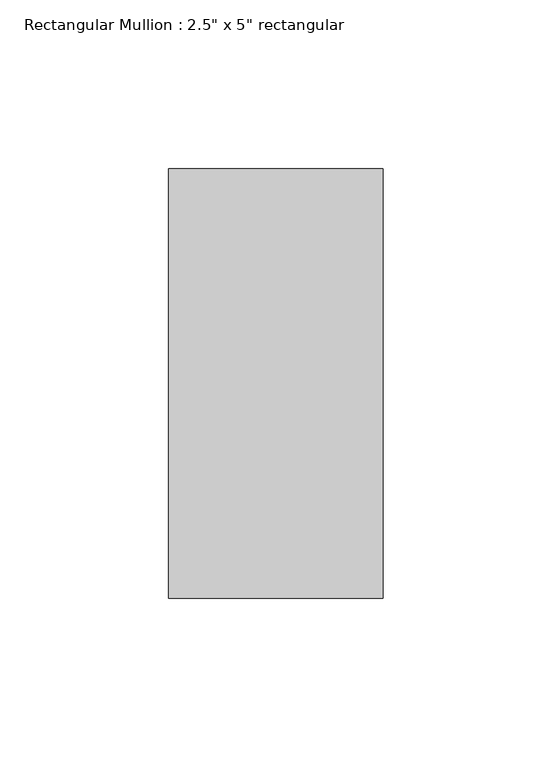
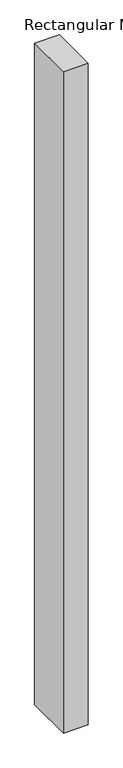
"""IFC4 building model written with IfcOpenShell, lengths in millimetres: member geometry."""

from ifc_helpers import new_model, si_unit, frame, origin, place, context, project, spatial, polyline, outline, extrude, source, transform, mapped, element, save


def member_89344730(model_context):
    return source(origin(), model_context, "Body", "SweptSolid", [
        extrude(outline(polyline([(0.0, 63.5), (0.0, -63.5), (-63.5, -63.5), (-63.5, 63.5), (0.0, 63.5)])), frame((0.0, 0.0, -1792.8537153), z_axis=(0.0, 0.0, 1.0), x_axis=(1.0, 0.0, 0.0)), (0.0, 0.0, 1.0), 1792.8537153),
    ])


if __name__ == "__main__":
    model = new_model("IFC4")
    model_context = context("Model", 3, world=origin())
    ifc_project = project(units=[si_unit("LENGTHUNIT", "METRE", prefix="MILLI")], contexts=[model_context])
    site = spatial("IfcSite", under=ifc_project)
    building = spatial("IfcBuilding", under=site)
    placement = place(None, origin())
    member_shape = member_89344730(model_context)
    element("IfcMember", 1, ObjectType="Rectangular Mullion : 2.5\" x 5\" rectangular", at=placement, inside=building, context=model_context, shape_type="MappedRepresentation", body=[
        mapped(member_shape, transform((0.0, 0.0, 0.0), x_axis=(1.0, 0.0, 0.0), y_axis=(0.0, 1.0, 0.0), z_axis=(0.0, 0.0, 1.0))),
    ])
    save(model, "model.ifc")

# Revit data of these elements
# Type "Rectangular Mullion : 2.5\" x 5\" rectangular"
#   built-in parameter 1007304 = 0.416667 (stored number, unit not read)
#   built-in parameter 1007301 = 0.104167 (stored number, unit not read)
#   built-in parameter 1007300 = 0.104167 (stored number, unit not read)
# Element 1 (IfcMember, "Rectangular Mullion : 2.5\" x 5\" rectangular")
#   Materials on its faces: "Aluminum"
# Materials
#   "Aluminum": class "Metal", colour RGB 247 247 247, transparency 0, Description = "Aluminum 6061", Cost = 0
